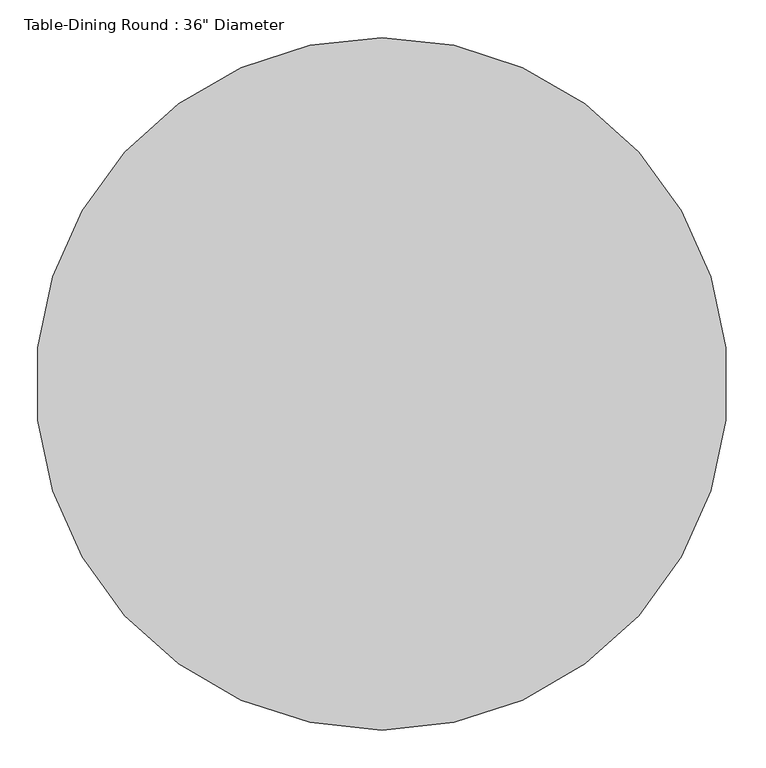
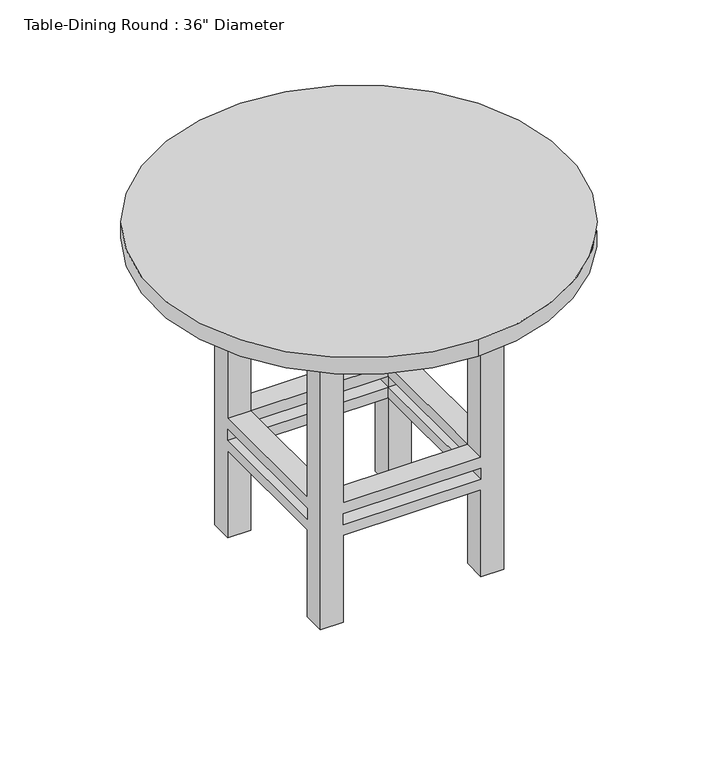
"""IFC4 building model written with IfcOpenShell, lengths in millimetres: furniture geometry."""

from ifc_helpers import new_model, si_unit, point, frame, frame_2d, origin, place, context, project, spatial, polyline, circle_curve, trimmed, segment, composite_curve, outline, extrude, faceted_brep, source, transform, mapped, element, save


def furniture_ec754799(model_context):
    return source(origin(), model_context, "Body", "SolidModel", [
        extrude(outline(polyline([(332.2819672, 43.7213115), (332.2819672, -413.4786885), (-124.9180328, -413.4786885), (-124.9180328, 43.7213115), (332.2819672, 43.7213115)]), holes=[polyline([(306.8819672, 18.3213115), (-99.5180328, 18.3213115), (-99.5180328, -388.0786885), (306.8819672, -388.0786885), (306.8819672, 18.3213115)])]), frame((0.0, 0.0, 647.7), z_axis=(0.0, 0.0, 1.0), x_axis=(1.0, 0.0, 0.0)), (0.0, 0.0, 1.0), 76.2),
        faceted_brep([(-48.7180328, 18.3213115, 723.9), (-99.5180328, 18.3213115, 723.9), (-99.5180328, -32.4786885, 723.9), (-48.7180328, -32.4786885, 723.9), (256.0819672, 18.3213115, 723.9), (256.0819672, -32.4786885, 723.9), (306.8819672, -32.4786885, 723.9), (306.8819672, 18.3213115, 723.9), (256.0819672, -388.0786885, 723.9), (306.8819672, -388.0786885, 723.9), (306.8819672, -337.2786885, 723.9), (256.0819672, -337.2786885, 723.9), (-48.7180328, -388.0786885, 723.9), (-48.7180328, -337.2786885, 723.9), (-99.5180328, -337.2786885, 723.9), (-99.5180328, -388.0786885, 723.9), (-48.7180328, 18.3213115, 0.0), (-48.7180328, -32.4786885, 0.0), (-99.5180328, -32.4786885, 0.0), (-99.5180328, 18.3213115, 0.0), (256.0819672, 18.3213115, 0.0), (306.8819672, 18.3213115, 0.0), (306.8819672, -32.4786885, 0.0), (256.0819672, -32.4786885, 0.0), (256.0819672, -388.0786885, 0.0), (256.0819672, -337.2786885, 0.0), (306.8819672, -337.2786885, 0.0), (306.8819672, -388.0786885, 0.0), (-48.7180328, -388.0786885, 0.0), (-99.5180328, -388.0786885, 0.0), (-99.5180328, -337.2786885, 0.0), (-48.7180328, -337.2786885, 0.0), (-48.7180328, 18.3213115, 279.4), (256.0819672, 18.3213115, 279.4), (256.0819672, 18.3213115, 203.2), (-48.7180328, 18.3213115, 203.2), (256.0819672, 18.3213115, 228.6), (256.0819672, 18.3213115, 254.0), (-48.7180328, 18.3213115, 254.0), (-48.7180328, 18.3213115, 228.6), (-99.5180328, -32.4786885, 203.2), (-99.5180328, -337.2786885, 203.2), (-99.5180328, -337.2786885, 279.4), (-99.5180328, -32.4786885, 279.4), (-99.5180328, -32.4786885, 228.6), (-99.5180328, -32.4786885, 254.0), (-99.5180328, -337.2786885, 254.0), (-99.5180328, -337.2786885, 228.6), (-48.7180328, -32.4786885, 279.4), (-48.7180328, -32.4786885, 203.2), (-48.7180328, -32.4786885, 228.6), (-48.7180328, -32.4786885, 254.0), (256.0819672, -32.4786885, 279.4), (256.0819672, -32.4786885, 203.2), (256.0819672, -32.4786885, 228.6), (256.0819672, -32.4786885, 254.0), (306.8819672, -32.4786885, 279.4), (306.8819672, -32.4786885, 203.2), (306.8819672, -32.4786885, 228.6), (306.8819672, -32.4786885, 254.0), (306.8819672, -337.2786885, 279.4), (306.8819672, -337.2786885, 203.2), (306.8819672, -337.2786885, 228.6), (306.8819672, -337.2786885, 254.0), (256.0819672, -388.0786885, 279.4), (-48.7180328, -388.0786885, 279.4), (-48.7180328, -388.0786885, 203.2), (256.0819672, -388.0786885, 203.2), (-48.7180328, -388.0786885, 228.6), (-48.7180328, -388.0786885, 254.0), (256.0819672, -388.0786885, 254.0), (256.0819672, -388.0786885, 228.6), (256.0819672, -337.2786885, 279.4), (256.0819672, -337.2786885, 203.2), (256.0819672, -337.2786885, 228.6), (256.0819672, -337.2786885, 254.0), (-48.7180328, -337.2786885, 279.4), (-48.7180328, -337.2786885, 203.2), (-48.7180328, -337.2786885, 228.6), (-48.7180328, -337.2786885, 254.0)], [[[0, 1, 2, 3]], [[4, 5, 6, 7]], [[8, 9, 10, 11]], [[12, 13, 14, 15]], [[16, 17, 18, 19]], [[20, 21, 22, 23]], [[24, 25, 26, 27]], [[28, 29, 30, 31]], [[1, 0, 32, 33, 4, 7, 21, 20, 34, 35, 16, 19], [36, 37, 38, 39]], [[2, 1, 19, 18, 40, 41, 30, 29, 15, 14, 42, 43], [44, 45, 46, 47]], [[3, 2, 43, 48]], [[18, 17, 49, 40]], [[44, 50, 51, 45]], [[0, 3, 48, 32]], [[17, 16, 35, 49]], [[50, 39, 38, 51]], [[5, 4, 33, 52]], [[20, 23, 53, 34]], [[36, 54, 55, 37]], [[6, 5, 52, 56]], [[23, 22, 57, 53]], [[54, 58, 59, 55]], [[21, 7, 6, 56, 60, 10, 9, 27, 26, 61, 57, 22], [62, 63, 59, 58]], [[27, 9, 8, 64, 65, 12, 15, 29, 28, 66, 67, 24], [68, 69, 70, 71]], [[11, 10, 60, 72]], [[26, 25, 73, 61]], [[62, 74, 75, 63]], [[8, 11, 72, 64]], [[25, 24, 67, 73]], [[74, 71, 70, 75]], [[13, 12, 65, 76]], [[28, 31, 77, 66]], [[68, 78, 79, 69]], [[14, 13, 76, 42]], [[31, 30, 41, 77]], [[78, 47, 46, 79]], [[54, 74, 62, 58]], [[74, 78, 68, 71]], [[78, 50, 44, 47]], [[50, 54, 36, 39]], [[53, 49, 35, 34]], [[49, 77, 41, 40]], [[77, 73, 67, 66]], [[73, 53, 57, 61]], [[74, 54, 53, 73]], [[78, 74, 73, 77]], [[50, 78, 77, 49]], [[54, 50, 49, 53]], [[52, 72, 60, 56]], [[72, 76, 65, 64]], [[76, 48, 43, 42]], [[48, 52, 33, 32]], [[55, 51, 38, 37]], [[51, 79, 46, 45]], [[79, 75, 70, 69]], [[75, 55, 59, 63]], [[72, 52, 55, 75]], [[76, 72, 75, 79]], [[48, 76, 79, 51]], [[52, 48, 51, 55]]]),
        extrude(outline(composite_curve([segment(trimmed(circle_curve(frame_2d((103.6819672, -184.8786885)), 457.2), [point((103.6819672, -642.0786885))], [point((103.6819672, 272.3213115))], False, "CARTESIAN"), True, "CONTINUOUS"), segment(trimmed(circle_curve(frame_2d((103.6819672, -184.8786885)), 457.2), [point((103.6819672, 272.3213115))], [point((103.6819672, -642.0786885))], False, "CARTESIAN"), True, "CONTINUOUS")], self_intersect=False)), frame((0.0, 0.0, 723.9), z_axis=(0.0, 0.0, 1.0), x_axis=(1.0, 0.0, 0.0)), (0.0, 0.0, 1.0), 38.1),
    ])


if __name__ == "__main__":
    model = new_model("IFC4")
    model_context = context("Model", 3, world=origin())
    ifc_project = project(units=[si_unit("LENGTHUNIT", "METRE", prefix="MILLI")], contexts=[model_context])
    site = spatial("IfcSite", under=ifc_project)
    building = spatial("IfcBuilding", under=site)
    placement = place(None, origin())
    furniture_shape = furniture_ec754799(model_context)
    element("IfcFurniture", 1, ObjectType="Table-Dining Round : 36\" Diameter", at=placement, inside=building, context=model_context, shape_type="MappedRepresentation", body=[
        mapped(furniture_shape, transform((0.0, 0.0, 0.0), x_axis=(1.0, 0.0, 0.0), y_axis=(0.0, 1.0, 0.0), z_axis=(0.0, 0.0, 1.0))),
    ])
    save(model, "model.ifc")

# Revit data of these elements
# Type "Table-Dining Round : 36\" Diameter"
#   Assembly Code = "E2020200"
#   Diameter = 3' - 0"
#   Height = 2' - 6"
#   Base Material = Pine
#   Top Material = Laminate, Linen, Matte
#   Default Elevation = 0
# Element 1 (IfcFurniture, "Table-Dining Round : 36\" Diameter")
#   Materials on its faces: "Pine", "Laminate, Linen, Matte"
# Materials
#   "Pine": class "Wood", colour RGB 223 192 134, transparency 0, Description = "Pinus Echinata", Cost = 0
#   "Laminate, Linen, Matte": class "Plastic", colour RGB 249 239 230, transparency 0, Description = "Plastic Laminate - Linen, Matte", Cost = 0
